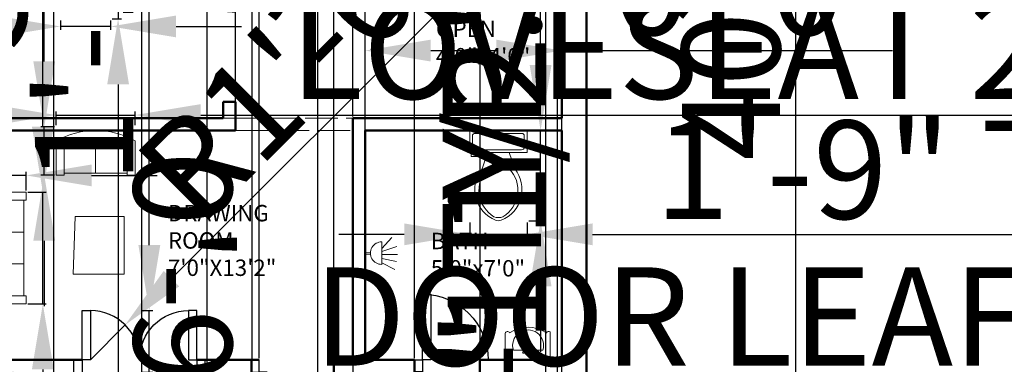
# Model space of a CAD drawing. Units: inches. Extents: x 1102 to 2414, y 295 to 1561.
# Tile 5 of 11: x 1610 to 1971, y 768 to 894. Entities that reach past the tile are written whole.
import ezdxf

# ---------------------------------------------------------------- set-up
doc = ezdxf.new("R2010")
doc.units = ezdxf.units.IN
doc.linetypes.add('ACAD_ISO02W100', pattern=[15, 12, -3])
for name, color, linetype, lineweight in [('A-ANNO-DIMS', 2, 'Continuous', 18), ('A-AREA-IDEN', 7, 'Continuous', 25), ('A-DOOR', 4, 'Continuous', 25), ('A-FLOR-FIXT', 9, 'Continuous', 18), ('A-FURN', 8, 'Continuous', 18), ('A-WALL', 7, 'Continuous', 50), ('A-WALL-OVHD', 7, 'ACAD_ISO02W100', 18)]:
    doc.layers.add(name, color=color, linetype=linetype, lineweight=lineweight)
doc.styles.get("Standard").update_dxf_attribs({"font": 'arial.ttf'})
doc.dimstyles.new('ISO-25', dxfattribs={"dimtxt": 36, "dimasz": 24, "dimexe": 1.25, "dimexo": 0.625, "dimtad": 1, "dimlunit": 4, "dimtxsty": 'Standard', "dimcen": 2.5, "dimadec": 0, "dimazin": 0, "dimtfac": 1, "dimtmove": 0, "dimatfit": 3, "dimfxl": 1, "dimarcsym": 0})

# ---------------------------------------------------------------- blocks, each defined once
blk = doc.blocks.new('*D3')
at = {"layer": 'A-ANNO-DIMS', "color": 0, "lineweight": -2, "transparency": 16777216}
for p, q in [((1818.17, 1116.76), (1895.42, 1116.76)), ((1894.17, 1092.76), (1894.17, 660.76)), ((1818.17, 636.76), (1895.42, 636.76))]:
    blk.add_line(p, q, dxfattribs=at)
at = {"layer": 'A-ANNO-DIMS', "color": 0, "transparency": 16777216}
for points in [[(1890.17, 1092.76), (1898.17, 1092.76), (1894.17, 1116.76)], [(1890.17, 660.76), (1898.17, 660.76), (1894.17, 636.76)]]:
    blk.add_solid(points, dxfattribs=at)
at = {"layer": 'Defpoints', "color": 0, "transparency": 16777216}
for p in [(1817.54, 1116.76), (1817.54, 636.76), (1894.17, 636.76)]:
    blk.add_point(p, dxfattribs=at)
at = {"layer": 'A-ANNO-DIMS', "color": 0, "transparency": 16777216, "insert": (1875.16, 876.76), "char_height": 36, "attachment_point": 5, "rotation": 90}
blk.add_mtext("40'", dxfattribs=at)
blk = doc.blocks.new('Sofa - Roundback 7 ft.')
for p, q in [((-12.00002, -32.4421), (-12.00003, -6.5971)), ((11.99997, -32.4421), (11.99998, -6.5971)), ((-36.000027, -34), (-36.000027, -11.4696)), ((-35.999844, -13.3819), (35.9998, -13.3819)), ((35.99998, -34), (35.99998, -11.4696)), ((-36.000027, -32.4421), (35.99998, -32.4421))]:
    blk.add_line(p, q)
for points in [[(-36.000027, -34), (-42.000027, -34), (-42.000027, -8)], [(41.99998, -8), (41.99998, -34), (35.99998, -34)]]:
    blk.add_lwpolyline(points)
for centre, radius, start, end in [((0, -114.25), 114.25, 68.43141, 111.5686), ((-0.00001, -127.1968), 121.1968, 72.72033, 107.2797)]:
    blk.add_arc(centre, radius, start, end)
blk = doc.blocks.new('Sofa - Roundback Loveseat 5 ft.')
for p, q in [((0, -32.44198), (0, -5.99998)), ((-24, -33.99998), (-24, -11.46958)), ((-23.9998, -13.38178), (23.99986, -13.38178)), ((24.00004, -33.99998), (24.00004, -11.46958)), ((-24, -32.44198), (24.00004, -32.44198))]:
    blk.add_line(p, q)
for points in [[(-24, -33.99998), (-30, -33.99998), (-30, -7.99998)], [(30.00004, -7.99998), (30.00004, -33.99998), (24.00004, -33.99998)]]:
    blk.add_lwpolyline(points)
for centre, radius, start, end in [((0, -60.24998), 60.24998, 60.13715, 119.8628), ((0, -61.38438), 55.38444, 64.32083, 115.6792)]:
    blk.add_arc(centre, radius, start, end)
blk = doc.blocks.new('Toilet - top')
for p, q in [((9.5, -6), (9.5, -2)), ((-10, -8.5), (-8, -8.5)), ((-10, -9.5), (-10, -8.5)), ((-7, -9.5), (-10, -9.5)), ((-8, -8.5), (-8, -8)), ((-7, -8), (-7, -9.5)), ((-4, -8), (-6, -14)), ((4, -8), (6, -14)), ((4, -14), (-4, -14))]:
    blk.add_line(p, q)
blk.add_lwpolyline([(10.5, -8), (10.5, 0), (-10.5, 0), (-10.5, -8)], close=True)
for points in [[(-9.5, -2), (-9.5, -6)], [(8.5, -1), (-8.5, -1)], [(-8.5, -7), (8.5, -7)]]:
    blk.add_lwpolyline(points)
for centre, radius, start, end in [((-8.62, -1.88), 0.884, 81.8699, 188.1301), ((8.62, -1.88), 0.884, 351.8699, 98.1301), ((-8.62, -6.12), 0.884, 171.8699, 278.1301), ((8.62, -6.12), 0.884, 261.8699, 8.1301), ((3.52, -21.58), 12.17, 141.4691, 247.9714), ((4.2, -21.82), 11.33, 136.3677, 238.9468), ((-3.52, -21.58), 12.17, 292.0284, 38.5307), ((-4.2, -21.82), 11.33, 301.053, 43.6321), ((0, -27.88), 4, 245.7318, 294.2682), ((0, -29), 4, 254.8605, 285.1395)]:
    blk.add_arc(centre, radius, start, end)
blk = doc.blocks.new('roomdoor')
for points in [[(1837.54, 1413.02), (1840.54, 1413.02), (1840.54, 1443.02), (1837.54, 1443.02)], [(1840.54, 1408.52), (1843.54, 1408.52), (1843.54, 1413.02), (1840.54, 1413.02)]]:
    blk.add_lwpolyline(points, close=True)
blk.add_arc((1840.54, 1413.02), 30, 90, 180)
blk = doc.blocks.new('utilitydoor')
for points in [[(1891.43, 1413.69), (1894.43, 1413.69), (1894.43, 1437.69), (1891.43, 1437.69)], [(1894.43, 1409.19), (1897.43, 1409.19), (1897.43, 1413.69), (1894.43, 1413.69)]]:
    blk.add_lwpolyline(points, close=True)
blk.add_arc((1894.43, 1413.69), 24, 90, 180)
blk = doc.blocks.new('DOOR-DOUBLE-LEAF-18')
blk.add_lwpolyline([(3, 22.5), (6, 22.5), (6, 4.5), (3, 4.5)], close=True)
blk.add_lwpolyline([(0, 0), (0, 4.5), (3, 4.5), (3, 0)])
blk.add_arc((6, 4.5), 18, 0, 90)
blk = doc.blocks.new('*D17')
at = {"layer": 'A-ANNO-DIMS', "color": 0, "lineweight": -2, "transparency": 16777216}
for p, q in [((1600.9, 891.85), (1102.3, 891.8)), ((1624.9, 893.98), (1624.9, 890.6)), ((1643.27, 891.85), (1624.9, 891.85)), ((1643.27, 893.98), (1643.27, 890.6)), ((1667.27, 891.85), (1691.27, 891.85))]:
    blk.add_line(p, q, dxfattribs=at)
at = {"layer": 'A-ANNO-DIMS', "color": 0, "transparency": 16777216}
for points in [[(1600.9, 895.85), (1600.9, 887.85), (1624.9, 891.85)], [(1667.27, 895.85), (1667.27, 887.85), (1643.27, 891.85)]]:
    blk.add_solid(points, dxfattribs=at)
at = {"layer": 'Defpoints', "color": 0, "transparency": 16777216}
for p in [(1624.9, 894.6), (1643.27, 894.6), (1624.9, 891.85)]:
    blk.add_point(p, dxfattribs=at)
at = {"layer": 'A-ANNO-DIMS', "color": 0, "transparency": 16777216, "insert": (1339.6, 911.06), "char_height": 36, "attachment_point": 5, "rotation": 0.0057}
blk.add_mtext('CHAIR 1\'-6 1/2" TYP.', dxfattribs=at)
blk = doc.blocks.new('*D18')
at = {"layer": 'A-ANNO-DIMS', "color": 0, "lineweight": -2, "transparency": 16777216}
for p, q in [((1646.02, 927.81), (1646.02, 951.81)), ((1643.89, 903.81), (1647.27, 903.81)), ((1646.02, 903.81), (1646.02, 894.61)), ((1643.89, 894.6), (1647.27, 894.61)), ((1646.03, 870.61), (1646.05, 625.92))]:
    blk.add_line(p, q, dxfattribs=at)
at = {"layer": 'A-ANNO-DIMS', "color": 0, "transparency": 16777216}
for points in [[(1650.02, 927.81), (1642.02, 927.81), (1646.02, 903.81)], [(1650.03, 870.61), (1642.03, 870.6), (1646.02, 894.61)]]:
    blk.add_solid(points, dxfattribs=at)
at = {"layer": 'Defpoints', "color": 0, "transparency": 16777216}
for p in [(1643.27, 903.81), (1643.27, 894.6), (1646.02, 894.61)]:
    blk.add_point(p, dxfattribs=at)
at = {"layer": 'A-ANNO-DIMS', "color": 0, "transparency": 16777216, "insert": (1665.05, 736.26), "char_height": 36, "attachment_point": 5, "rotation": 270.0057}
blk.add_mtext('0\'-9" TYP.', dxfattribs=at)
blk = doc.blocks.new('*D20')
at = {"layer": 'A-ANNO-DIMS', "color": 0, "lineweight": -2, "transparency": 16777216}
for p, q in [((1808.58, 695.77), (1808.58, 1020.95)), ((1806.65, 671.77), (1809.83, 671.77)), ((1808.58, 658.48), (1808.58, 671.77)), ((1806.65, 658.48), (1809.83, 658.48)), ((1808.58, 634.48), (1808.58, 610.48))]:
    blk.add_line(p, q, dxfattribs=at)
at = {"layer": 'A-ANNO-DIMS', "color": 0, "transparency": 16777216}
for points in [[(1804.58, 695.77), (1812.58, 695.77), (1808.58, 671.77)], [(1804.58, 634.48), (1812.58, 634.48), (1808.58, 658.48)]]:
    blk.add_solid(points, dxfattribs=at)
at = {"layer": 'Defpoints', "color": 0, "transparency": 16777216}
for p in [(1806.03, 671.77), (1808.58, 671.77), (1806.03, 658.48)]:
    blk.add_point(p, dxfattribs=at)
at = {"layer": 'A-ANNO-DIMS', "color": 0, "transparency": 16777216, "insert": (1789.34, 870.36), "char_height": 36, "attachment_point": 5, "rotation": 90}
blk.add_mtext('1\'-1 1/2" TYP.', dxfattribs=at)
blk = doc.blocks.new('*D21')
at = {"layer": 'A-ANNO-DIMS', "color": 0, "lineweight": -2, "transparency": 16777216}
for p, q in [((1731.22, 677.69), (1731.22, 665.84)), ((1806.03, 677.69), (1806.03, 665.84)), ((1755.22, 667.09), (1782.03, 667.09)), ((1806.03, 667.09), (2237.1, 667.09))]:
    blk.add_line(p, q, dxfattribs=at)
at = {"layer": 'A-ANNO-DIMS', "color": 0, "transparency": 16777216}
for points in [[(1755.22, 671.09), (1755.22, 663.09), (1731.22, 667.09)], [(1782.03, 671.09), (1782.03, 663.09), (1806.03, 667.09)]]:
    blk.add_solid(points, dxfattribs=at)
at = {"layer": 'Defpoints', "color": 0, "transparency": 16777216}
for p in [(1731.22, 678.32), (1806.03, 678.32), (1806.03, 667.09)]:
    blk.add_point(p, dxfattribs=at)
at = {"layer": 'A-ANNO-DIMS', "color": 0, "transparency": 16777216, "insert": (2033.56, 687.44), "char_height": 36, "attachment_point": 5}
blk.add_mtext('QUEEN BED 6\'-3"', dxfattribs=at)
blk = doc.blocks.new('*D24')
at = {"layer": 'A-ANNO-DIMS', "color": 0, "lineweight": -2, "transparency": 16777216}
for p, q in [((1725.17, 1080.27), (1712.37, 1080.27)), ((1713.62, 1056.27), (1713.62, 1043.39)), ((1725.17, 1019.39), (1712.37, 1019.39)), ((1713.62, 1019.39), (1713.62, 898.44))]:
    blk.add_line(p, q, dxfattribs=at)
at = {"layer": 'A-ANNO-DIMS', "color": 0, "transparency": 16777216}
for points in [[(1709.62, 1056.27), (1717.62, 1056.27), (1713.62, 1080.27)], [(1709.62, 1043.39), (1717.62, 1043.39), (1713.62, 1019.39)]]:
    blk.add_solid(points, dxfattribs=at)
at = {"layer": 'Defpoints', "color": 0, "transparency": 16777216}
for p in [(1725.8, 1080.27), (1713.62, 1019.39), (1725.8, 1019.39)]:
    blk.add_point(p, dxfattribs=at)
at = {"layer": 'A-ANNO-DIMS', "color": 0, "transparency": 16777216, "insert": (1694.62, 946.91), "char_height": 36, "attachment_point": 5, "rotation": 90}
blk.add_mtext('5\'-1"', dxfattribs=at)
blk = doc.blocks.new('*D25')
at = {"layer": 'A-ANNO-DIMS', "color": 0, "lineweight": -2, "transparency": 16777216}
for p, q in [((1800.76, 877.69), (1800.76, 1221.61)), ((1796.43, 853.69), (1802.01, 853.69)), ((1800.76, 820.65), (1800.76, 853.69)), ((1796.43, 820.65), (1802.01, 820.65)), ((1800.76, 796.65), (1800.76, 772.65))]:
    blk.add_line(p, q, dxfattribs=at)
at = {"layer": 'A-ANNO-DIMS', "color": 0, "transparency": 16777216}
for points in [[(1796.76, 877.69), (1804.76, 877.69), (1800.76, 853.69)], [(1796.76, 796.65), (1804.76, 796.65), (1800.76, 820.65)]]:
    blk.add_solid(points, dxfattribs=at)
at = {"layer": 'Defpoints', "color": 0, "transparency": 16777216}
for p in [(1795.81, 853.69), (1800.76, 853.69), (1795.81, 820.65)]:
    blk.add_point(p, dxfattribs=at)
at = {"layer": 'A-ANNO-DIMS', "color": 0, "transparency": 16777216, "insert": (1781.53, 1061.65), "char_height": 36, "attachment_point": 5, "rotation": 90}
blk.add_mtext('WC 2\'-9" TYP.', dxfattribs=at)
blk = doc.blocks.new('*D26')
at = {"layer": 'A-ANNO-DIMS', "color": 0, "lineweight": -2, "transparency": 16777216}
for p, q in [((1774.81, 820.02), (1774.81, 814.44)), ((1795.81, 820.02), (1795.81, 814.44)), ((1750.81, 815.69), (1726.81, 815.69)), ((1774.81, 815.69), (1795.81, 815.69)), ((1819.81, 815.69), (2061.11, 815.69))]:
    blk.add_line(p, q, dxfattribs=at)
at = {"layer": 'A-ANNO-DIMS', "color": 0, "transparency": 16777216}
for points in [[(1750.81, 819.69), (1750.81, 811.69), (1774.81, 815.69)], [(1819.81, 819.69), (1819.81, 811.69), (1795.81, 815.69)]]:
    blk.add_solid(points, dxfattribs=at)
at = {"layer": 'Defpoints', "color": 0, "transparency": 16777216}
for p in [(1774.81, 820.65), (1795.81, 820.65), (1795.81, 815.69)]:
    blk.add_point(p, dxfattribs=at)
at = {"layer": 'A-ANNO-DIMS', "color": 0, "transparency": 16777216, "insert": (1952.46, 834.69), "char_height": 36, "attachment_point": 5}
blk.add_mtext('1\'-9" TYP.', dxfattribs=at)
blk = doc.blocks.new('*D29')
at = {"layer": 'A-ANNO-DIMS', "color": 0, "lineweight": -2, "transparency": 16777216}
for p, q in [((1806.82, 1011.76), (1806.82, 1035.76)), ((1803.17, 987.76), (1808.07, 987.76)), ((1806.82, 987.76), (1806.82, 959.26)), ((1803.17, 959.26), (1808.07, 959.26)), ((1806.82, 935.26), (1806.82, 295.33))]:
    blk.add_line(p, q, dxfattribs=at)
at = {"layer": 'A-ANNO-DIMS', "color": 0, "transparency": 16777216}
for points in [[(1802.82, 1011.76), (1810.82, 1011.76), (1806.82, 987.76)], [(1802.82, 935.26), (1810.82, 935.26), (1806.82, 959.26)]]:
    blk.add_solid(points, dxfattribs=at)
at = {"layer": 'Defpoints', "color": 0, "transparency": 16777216}
for p in [(1802.54, 987.76), (1802.54, 959.26), (1806.82, 959.26)]:
    blk.add_point(p, dxfattribs=at)
at = {"layer": 'A-ANNO-DIMS', "color": 0, "transparency": 16777216, "insert": (1787.57, 603.3), "char_height": 36, "attachment_point": 5, "rotation": 90}
blk.add_mtext('BATH DOOR 2\'-4 1/2" TYP.', dxfattribs=at)
blk = doc.blocks.new('*D31')
at = {"layer": 'A-ANNO-DIMS', "color": 0, "lineweight": -2, "transparency": 16777216}
for p, q in [((1629.86, 764.63), (1629.86, 760.41)), ((1653.86, 764.63), (1653.86, 760.41)), ((1605.86, 761.66), (1581.86, 761.66)), ((1629.86, 761.66), (1653.86, 761.66)), ((1677.86, 761.66), (2225.36, 761.66))]:
    blk.add_line(p, q, dxfattribs=at)
at = {"layer": 'A-ANNO-DIMS', "color": 0, "transparency": 16777216}
for points in [[(1605.86, 765.66), (1605.86, 757.66), (1629.86, 761.66)], [(1677.86, 765.66), (1677.86, 757.66), (1653.86, 761.66)]]:
    blk.add_solid(points, dxfattribs=at)
at = {"layer": 'Defpoints', "color": 0, "transparency": 16777216}
for p in [(1629.86, 765.26), (1653.86, 765.26), (1653.86, 761.66)]:
    blk.add_point(p, dxfattribs=at)
at = {"layer": 'A-ANNO-DIMS', "color": 0, "transparency": 16777216, "insert": (1963.61, 780.91), "char_height": 36, "attachment_point": 5}
blk.add_mtext('DOOR LEAF 2\'-0" TYP.', dxfattribs=at)
blk = doc.blocks.new('*D32')
at = {"layer": 'A-ANNO-DIMS', "color": 0, "lineweight": -2, "transparency": 16777216}
for p, q in [((1657.46, 811.76), (1657.46, 1164.91)), ((1654.49, 787.76), (1658.71, 787.76)), ((1657.46, 765.26), (1657.46, 787.76)), ((1654.49, 765.26), (1658.71, 765.26)), ((1657.46, 741.26), (1657.46, 717.26))]:
    blk.add_line(p, q, dxfattribs=at)
at = {"layer": 'A-ANNO-DIMS', "color": 0, "transparency": 16777216}
for points in [[(1653.46, 811.76), (1661.46, 811.76), (1657.46, 787.76)], [(1653.46, 741.26), (1661.46, 741.26), (1657.46, 765.26)]]:
    blk.add_solid(points, dxfattribs=at)
at = {"layer": 'Defpoints', "color": 0, "transparency": 16777216}
for p in [(1653.86, 787.76), (1657.46, 787.76), (1653.86, 765.26)]:
    blk.add_point(p, dxfattribs=at)
at = {"layer": 'A-ANNO-DIMS', "color": 0, "transparency": 16777216, "insert": (1638.22, 1000.34), "char_height": 36, "attachment_point": 5, "rotation": 90}
blk.add_mtext('1\'-10 1/2" TYP.', dxfattribs=at)
blk = doc.blocks.new('*D37')
at = {"layer": 'A-ANNO-DIMS', "color": 0, "lineweight": -2, "transparency": 16777216}
for p, q in [((1618.46, 855.15), (1618.46, 1126.82)), ((1612.94, 831.15), (1619.71, 831.15)), ((1618.46, 790.23), (1618.46, 831.15)), ((1612.94, 790.23), (1619.71, 790.23)), ((1618.46, 766.23), (1618.46, 742.23))]:
    blk.add_line(p, q, dxfattribs=at)
at = {"layer": 'A-ANNO-DIMS', "color": 0, "transparency": 16777216}
for points in [[(1614.46, 855.15), (1622.46, 855.15), (1618.46, 831.15)], [(1614.46, 766.23), (1622.46, 766.23), (1618.46, 790.23)]]:
    blk.add_solid(points, dxfattribs=at)
at = {"layer": 'Defpoints', "color": 0, "transparency": 16777216}
for p in [(1612.32, 831.15), (1618.46, 831.15), (1612.32, 790.23)]:
    blk.add_point(p, dxfattribs=at)
at = {"layer": 'A-ANNO-DIMS', "color": 0, "transparency": 16777216, "insert": (1599.19, 1002.98), "char_height": 36, "attachment_point": 5, "rotation": 90}
blk.add_mtext('SOFA 3\'-5"', dxfattribs=at)
blk = doc.blocks.new('*D38')
at = {"layer": 'A-ANNO-DIMS', "color": 0, "lineweight": -2, "transparency": 16777216}
for p, q in [((1570.46, 837.28), (1452.9, 837.28)), ((1594.46, 831.77), (1594.46, 838.53)), ((1612.32, 837.28), (1594.46, 837.28)), ((1612.32, 831.77), (1612.32, 838.53)), ((1636.32, 837.28), (1660.32, 837.28))]:
    blk.add_line(p, q, dxfattribs=at)
at = {"layer": 'A-ANNO-DIMS', "color": 0, "transparency": 16777216}
for points in [[(1570.46, 841.28), (1570.46, 833.28), (1594.46, 837.28)], [(1636.32, 841.28), (1636.32, 833.28), (1612.32, 837.28)]]:
    blk.add_solid(points, dxfattribs=at)
at = {"layer": 'Defpoints', "color": 0, "transparency": 16777216}
for p in [(1594.46, 837.28), (1594.46, 831.15), (1612.32, 831.15)]:
    blk.add_point(p, dxfattribs=at)
at = {"layer": 'A-ANNO-DIMS', "color": 0, "transparency": 16777216, "insert": (1499.68, 856.29), "char_height": 36, "attachment_point": 5}
blk.add_mtext('1\'-6"', dxfattribs=at)
blk = doc.blocks.new('*D39')
at = {"layer": 'A-ANNO-DIMS', "color": 0, "lineweight": -2, "transparency": 16777216}
for p, q in [((1599.32, 859.39), (1575.32, 859.39)), ((1623.32, 855.67), (1623.32, 860.64)), ((1623.32, 859.39), (1652.27, 859.39)), ((1652.27, 855.67), (1652.27, 860.64)), ((1676.27, 859.39), (2075.12, 859.39))]:
    blk.add_line(p, q, dxfattribs=at)
at = {"layer": 'A-ANNO-DIMS', "color": 0, "transparency": 16777216}
for points in [[(1599.32, 863.39), (1599.32, 855.39), (1623.32, 859.39)], [(1676.27, 863.39), (1676.27, 855.39), (1652.27, 859.39)]]:
    blk.add_solid(points, dxfattribs=at)
at = {"layer": 'Defpoints', "color": 0, "transparency": 16777216}
for p in [(1652.27, 859.39), (1623.32, 855.05), (1652.27, 855.05)]:
    blk.add_point(p, dxfattribs=at)
at = {"layer": 'A-ANNO-DIMS', "color": 0, "transparency": 16777216, "insert": (1887.69, 878.64), "char_height": 36, "attachment_point": 5}
blk.add_mtext('LOVESEAT 2\'-5"', dxfattribs=at)
blk = doc.blocks.new('*D40')
at = {"layer": 'A-ANNO-DIMS', "color": 0, "lineweight": -2, "transparency": 16777216}
for p, q in [((1618.98, 879.05), (1618.98, 1080.49)), ((1622.7, 855.05), (1617.73, 855.05)), ((1618.98, 837.36), (1618.98, 855.05)), ((1622.7, 837.36), (1617.73, 837.36)), ((1618.98, 813.36), (1618.98, 789.36))]:
    blk.add_line(p, q, dxfattribs=at)
at = {"layer": 'A-ANNO-DIMS', "color": 0, "transparency": 16777216}
for points in [[(1614.98, 879.05), (1622.98, 879.05), (1618.98, 855.05)], [(1614.98, 813.36), (1622.98, 813.36), (1618.98, 837.36)]]:
    blk.add_solid(points, dxfattribs=at)
at = {"layer": 'Defpoints', "color": 0, "transparency": 16777216}
for p in [(1618.98, 855.05), (1623.32, 855.05), (1623.32, 837.36)]:
    blk.add_point(p, dxfattribs=at)
at = {"layer": 'A-ANNO-DIMS', "color": 0, "transparency": 16777216, "insert": (1599.74, 991.77), "char_height": 36, "attachment_point": 5, "rotation": 90}
blk.add_mtext('1\'-5 1/2"', dxfattribs=at)
blk = doc.blocks.new('*D45')
at = {"layer": 'A-ANNO-DIMS', "color": 0, "lineweight": -2, "transparency": 16777216}
for p, q in [((1736.54, 770.38), (1736.54, 1147.26)), ((1754.54, 770.38), (1754.54, 1147.26)), ((1712.54, 1146.01), (1688.54, 1146.01)), ((1736.54, 1146.01), (1754.54, 1146.01)), ((1778.54, 1146.01), (1896.1, 1146.01))]:
    blk.add_line(p, q, dxfattribs=at)
at = {"layer": 'A-ANNO-DIMS', "color": 0, "transparency": 16777216}
for points in [[(1712.54, 1150.01), (1712.54, 1142.01), (1736.54, 1146.01)], [(1778.54, 1150.01), (1778.54, 1142.01), (1754.54, 1146.01)]]:
    blk.add_solid(points, dxfattribs=at)
at = {"layer": 'Defpoints', "color": 0, "transparency": 16777216}
for p in [(1754.54, 1146.01), (1736.54, 769.76), (1754.54, 769.76)]:
    blk.add_point(p, dxfattribs=at)
at = {"layer": 'A-ANNO-DIMS', "color": 0, "transparency": 16777216, "insert": (1849.32, 1165.02), "char_height": 36, "attachment_point": 5}
blk.add_mtext('1\'-6"', dxfattribs=at)
blk = doc.blocks.new('*D46')
at = {"layer": 'A-ANNO-DIMS', "color": 0, "lineweight": -2, "transparency": 16777216}
for p, q in [((1732.04, 857.63), (1732.04, 606.26)), ((1586.54, 853.13), (1586.54, 606.26)), ((1610.54, 607.51), (1708.04, 607.51)), ((1732.04, 607.51), (1961.46, 607.51))]:
    blk.add_line(p, q, dxfattribs=at)
at = {"layer": 'A-ANNO-DIMS', "color": 0, "transparency": 16777216}
for points in [[(1610.54, 611.51), (1610.54, 603.51), (1586.54, 607.51)], [(1708.04, 611.51), (1708.04, 603.51), (1732.04, 607.51)]]:
    blk.add_solid(points, dxfattribs=at)
at = {"layer": 'Defpoints', "color": 0, "transparency": 16777216}
for p in [(1732.04, 858.26), (1586.54, 853.76), (1732.04, 607.51)]:
    blk.add_point(p, dxfattribs=at)
at = {"layer": 'A-ANNO-DIMS', "color": 0, "transparency": 16777216, "insert": (1858.75, 626.75), "char_height": 36, "attachment_point": 5}
blk.add_mtext('12\'-1 1/2"', dxfattribs=at)
blk = doc.blocks.new('*D47')
at = {"layer": 'A-ANNO-DIMS', "color": 0, "lineweight": -2, "transparency": 16777216}
for p, q in [((1736.54, 854.38), (1736.54, 884.26)), ((1808.54, 854.38), (1808.54, 884.26)), ((1760.54, 883.01), (1784.54, 883.01)), ((1808.54, 883.01), (1929.69, 883.01))]:
    blk.add_line(p, q, dxfattribs=at)
at = {"layer": 'A-ANNO-DIMS', "color": 0, "transparency": 16777216}
for points in [[(1760.54, 887.01), (1760.54, 879.01), (1736.54, 883.01)], [(1784.54, 887.01), (1784.54, 879.01), (1808.54, 883.01)]]:
    blk.add_solid(points, dxfattribs=at)
at = {"layer": 'Defpoints', "color": 0, "transparency": 16777216}
for p in [(1808.54, 883.01), (1736.54, 853.76), (1808.54, 853.76)]:
    blk.add_point(p, dxfattribs=at)
at = {"layer": 'A-ANNO-DIMS', "color": 0, "transparency": 16777216, "insert": (1881.12, 902.02), "char_height": 36, "attachment_point": 5}
blk.add_mtext('6\'-0"', dxfattribs=at)
blk = doc.blocks.new('*D48')
at = {"layer": 'A-ANNO-DIMS', "color": 0, "lineweight": -2, "transparency": 16777216}
for p, q in [((1689.04, 854.38), (1689.04, 1147.26)), ((1732.04, 858.88), (1732.04, 1147.26)), ((1665.04, 1146.01), (1641.04, 1146.01)), ((1689.04, 1146.01), (1732.04, 1146.01)), ((1756.04, 1146.01), (1876.97, 1146.01))]:
    blk.add_line(p, q, dxfattribs=at)
at = {"layer": 'A-ANNO-DIMS', "color": 0, "transparency": 16777216}
for points in [[(1665.04, 1150.01), (1665.04, 1142.01), (1689.04, 1146.01)], [(1756.04, 1150.01), (1756.04, 1142.01), (1732.04, 1146.01)]]:
    blk.add_solid(points, dxfattribs=at)
at = {"layer": 'Defpoints', "color": 0, "transparency": 16777216}
for p in [(1732.04, 1146.01), (1732.04, 858.26), (1689.04, 853.76)]:
    blk.add_point(p, dxfattribs=at)
at = {"layer": 'A-ANNO-DIMS', "color": 0, "transparency": 16777216, "insert": (1828.51, 1165.03), "char_height": 36, "attachment_point": 5}
blk.add_mtext('3\'-7"', dxfattribs=at)
blk = doc.blocks.new('*D50')
at = {"layer": 'A-ANNO-DIMS', "color": 0, "lineweight": -2, "transparency": 16777216}
for p, q in [((1586.54, 987.13), (1586.54, 606.26)), ((1654.54, 987.13), (1654.54, 606.26)), ((1610.54, 607.51), (1630.54, 607.51)), ((1654.54, 607.51), (1775.49, 607.51))]:
    blk.add_line(p, q, dxfattribs=at)
at = {"layer": 'A-ANNO-DIMS', "color": 0, "transparency": 16777216}
for points in [[(1610.54, 611.51), (1610.54, 603.51), (1586.54, 607.51)], [(1630.54, 611.51), (1630.54, 603.51), (1654.54, 607.51)]]:
    blk.add_solid(points, dxfattribs=at)
at = {"layer": 'Defpoints', "color": 0, "transparency": 16777216}
for p in [(1586.54, 987.76), (1654.54, 987.76), (1654.54, 607.51)]:
    blk.add_point(p, dxfattribs=at)
at = {"layer": 'A-ANNO-DIMS', "color": 0, "transparency": 16777216, "insert": (1727.02, 626.52), "char_height": 36, "attachment_point": 5}
blk.add_mtext('5\'-8"', dxfattribs=at)
blk = doc.blocks.new('*D55')
at = {"layer": 'A-ANNO-DIMS', "color": 0, "lineweight": -2, "transparency": 16777216}
for p, q in [((1586.54, 722.38), (1586.54, 1147.26)), ((1622.54, 722.38), (1622.54, 1147.26)), ((1562.54, 1146.01), (1538.54, 1146.01)), ((1586.54, 1146.01), (1622.54, 1146.01)), ((1646.54, 1146.01), (1767.47, 1146.01))]:
    blk.add_line(p, q, dxfattribs=at)
at = {"layer": 'A-ANNO-DIMS', "color": 0, "transparency": 16777216}
for points in [[(1562.54, 1150.01), (1562.54, 1142.01), (1586.54, 1146.01)], [(1646.54, 1150.01), (1646.54, 1142.01), (1622.54, 1146.01)]]:
    blk.add_solid(points, dxfattribs=at)
at = {"layer": 'Defpoints', "color": 0, "transparency": 16777216}
for p in [(1622.54, 1146.01), (1586.54, 721.76), (1622.54, 721.76)]:
    blk.add_point(p, dxfattribs=at)
at = {"layer": 'A-ANNO-DIMS', "color": 0, "transparency": 16777216, "insert": (1719.01, 1165.03), "char_height": 36, "attachment_point": 5}
blk.add_mtext('3\'-0"', dxfattribs=at)
blk = doc.blocks.new('*D59')
at = {"layer": 'A-ANNO-DIMS', "color": 0, "lineweight": -2, "transparency": 16777216}
for p, q in [((1548.29, 962.66), (1548.29, 1112.19)), ((1612.15, 938.66), (1547.04, 938.66)), ((1548.29, 903.8), (1548.29, 938.66)), ((1612.15, 903.8), (1547.04, 903.8)), ((1548.29, 879.8), (1548.29, 855.8))]:
    blk.add_line(p, q, dxfattribs=at)
at = {"layer": 'A-ANNO-DIMS', "color": 0, "transparency": 16777216}
for points in [[(1544.29, 962.66), (1552.29, 962.66), (1548.29, 938.66)], [(1544.29, 879.8), (1552.29, 879.8), (1548.29, 903.8)]]:
    blk.add_solid(points, dxfattribs=at)
at = {"layer": 'Defpoints', "color": 0, "transparency": 16777216}
for p in [(1548.29, 938.66), (1612.78, 938.66), (1612.78, 903.8)]:
    blk.add_point(p, dxfattribs=at)
at = {"layer": 'A-ANNO-DIMS', "color": 0, "transparency": 16777216, "insert": (1529.6, 1049.43), "char_height": 36, "attachment_point": 5, "rotation": 90}
blk.add_mtext('2\'-11"', dxfattribs=at)
blk = doc.blocks.new('*D62')
at = {"layer": 'A-ANNO-DIMS', "color": 0, "lineweight": -2, "transparency": 16777216}
for p, q in [((1778.54, 982.63), (1778.54, 606.26)), ((1802.54, 982.63), (1802.54, 606.26)), ((1754.54, 607.51), (1730.54, 607.51)), ((1778.54, 607.51), (1802.54, 607.51)), ((1826.54, 607.51), (1948.11, 607.51))]:
    blk.add_line(p, q, dxfattribs=at)
at = {"layer": 'A-ANNO-DIMS', "color": 0, "transparency": 16777216}
for points in [[(1754.54, 611.51), (1754.54, 603.51), (1778.54, 607.51)], [(1826.54, 611.51), (1826.54, 603.51), (1802.54, 607.51)]]:
    blk.add_solid(points, dxfattribs=at)
at = {"layer": 'Defpoints', "color": 0, "transparency": 16777216}
for p in [(1778.54, 983.26), (1802.54, 983.26), (1802.54, 607.51)]:
    blk.add_point(p, dxfattribs=at)
at = {"layer": 'A-ANNO-DIMS', "color": 0, "transparency": 16777216, "insert": (1899.32, 626.52), "char_height": 36, "attachment_point": 5}
blk.add_mtext('2\'-0"', dxfattribs=at)
blk = doc.blocks.new('*D63')
at = {"layer": 'A-ANNO-DIMS', "color": 0, "lineweight": -2, "transparency": 16777216}
for p, q in [((1654.54, 982.63), (1654.54, 606.26)), ((1678.54, 982.63), (1678.54, 606.26)), ((1630.54, 607.51), (1606.54, 607.51)), ((1654.54, 607.51), (1678.54, 607.51)), ((1702.54, 607.51), (1824.11, 607.51))]:
    blk.add_line(p, q, dxfattribs=at)
at = {"layer": 'A-ANNO-DIMS', "color": 0, "transparency": 16777216}
for points in [[(1630.54, 611.51), (1630.54, 603.51), (1654.54, 607.51)], [(1702.54, 611.51), (1702.54, 603.51), (1678.54, 607.51)]]:
    blk.add_solid(points, dxfattribs=at)
at = {"layer": 'Defpoints', "color": 0, "transparency": 16777216}
for p in [(1654.54, 983.26), (1678.54, 983.26), (1678.54, 607.51)]:
    blk.add_point(p, dxfattribs=at)
at = {"layer": 'A-ANNO-DIMS', "color": 0, "transparency": 16777216, "insert": (1775.32, 626.52), "char_height": 36, "attachment_point": 5}
blk.add_mtext('2\'-0"', dxfattribs=at)
blk = doc.blocks.new('*D64')
at = {"layer": 'A-ANNO-DIMS', "color": 0, "lineweight": -2, "transparency": 16777216}
for p, q in [((1695.04, 982.63), (1695.04, 606.26)), ((1719.04, 982.63), (1719.04, 606.26)), ((1671.04, 607.51), (1647.04, 607.51)), ((1695.04, 607.51), (1719.04, 607.51)), ((1743.04, 607.51), (1864.61, 607.51))]:
    blk.add_line(p, q, dxfattribs=at)
at = {"layer": 'A-ANNO-DIMS', "color": 0, "transparency": 16777216}
for points in [[(1671.04, 611.51), (1671.04, 603.51), (1695.04, 607.51)], [(1743.04, 611.51), (1743.04, 603.51), (1719.04, 607.51)]]:
    blk.add_solid(points, dxfattribs=at)
at = {"layer": 'Defpoints', "color": 0, "transparency": 16777216}
for p in [(1695.04, 983.26), (1719.04, 983.26), (1719.04, 607.51)]:
    blk.add_point(p, dxfattribs=at)
at = {"layer": 'A-ANNO-DIMS', "color": 0, "transparency": 16777216, "insert": (1815.82, 626.52), "char_height": 36, "attachment_point": 5}
blk.add_mtext('2\'-0"', dxfattribs=at)
blk = doc.blocks.new('*D65')
at = {"layer": 'A-ANNO-DIMS', "color": 0, "lineweight": -2, "transparency": 16777216}
for p, q in [((1697.64, 770.38), (1697.64, 1147.26)), ((1725.04, 770.38), (1725.04, 1147.26)), ((1673.64, 1146.01), (1649.64, 1146.01)), ((1697.64, 1146.01), (1725.04, 1146.01)), ((1749.04, 1146.01), (1954.49, 1146.01))]:
    blk.add_line(p, q, dxfattribs=at)
at = {"layer": 'A-ANNO-DIMS', "color": 0, "transparency": 16777216}
for points in [[(1673.64, 1150.01), (1673.64, 1142.01), (1697.64, 1146.01)], [(1749.04, 1150.01), (1749.04, 1142.01), (1725.04, 1146.01)]]:
    blk.add_solid(points, dxfattribs=at)
at = {"layer": 'Defpoints', "color": 0, "transparency": 16777216}
for p in [(1725.04, 1146.01), (1697.64, 769.76), (1725.04, 769.76)]:
    blk.add_point(p, dxfattribs=at)
at = {"layer": 'A-ANNO-DIMS', "color": 0, "transparency": 16777216, "insert": (1863.77, 1165.26), "char_height": 36, "attachment_point": 5}
blk.add_mtext('2\'-3 1/2"', dxfattribs=at)
blk = doc.blocks.new('*D69')
at = {"layer": 'A-ANNO-DIMS', "color": 0, "lineweight": -2, "transparency": 16777216}
for p, q in [((1775.45, 909.34), (1665.56, 799.46)), ((1635.86, 769.76), (1648.59, 782.49))]:
    blk.add_line(p, q, dxfattribs=at)
at = {"layer": 'A-ANNO-DIMS', "color": 0, "transparency": 16777216}
blk.add_solid([(1662.73, 802.29), (1668.39, 796.63), (1648.59, 782.49)], dxfattribs=at)
at = {"layer": 'Defpoints', "color": 0, "transparency": 16777216}
for p in [(1648.59, 782.49), (1635.86, 769.76)]:
    blk.add_point(p, dxfattribs=at)
at = {"layer": 'A-ANNO-DIMS', "color": 0, "transparency": 16777216, "insert": (1715.55, 876.32), "char_height": 36, "attachment_point": 5, "rotation": 45}
blk.add_mtext('R1\'-6"', dxfattribs=at)

msp = doc.modelspace()

# ---------------------------------------------------------------- linework, layer by layer
at = {"layer": 'A-FLOR-FIXT'}
for p, q in [((1742.618, 810.56), (1746.255, 814.541)), ((1742.618, 812.925), (1742.618, 804.685)), ((1736.544, 808.967), (1738.415, 808.917)), ((1736.544, 808.33), (1738.426, 808.48)), ((1742.618, 809.445), (1748.136, 811.293)), ((1742.618, 808.362), (1748.359, 808.33)), ((1742.618, 806.865), (1748.009, 805.687)), ((1742.618, 805.273), (1747.339, 802.82)), ((1787.777, 769.76), (1787.777, 779.467)), ((1804.289, 769.76), (1804.289, 779.929)), ((1790.827, 773.205), (1801.552, 773.205)), ((1787.777, 769.76), (1804.289, 769.76))]:
    msp.add_line(p, q, dxfattribs=at)
for centre, radius in [((1794.411, 772.402), 0.284), ((1796.037, 774.2), 0.461), ((1796.032, 772.706), 0.365), ((1797.572, 772.199), 0.324)]:
    msp.add_circle(centre, radius, dxfattribs=at)
for centre, radius, start, end in [((1742.534, 808.805), 4.121, 88.83988, 271.16012), ((1788.596, 779.214), 0.857, 25.5147, 162.79987), ((1796.17, 769.344), 12.292, 56.40939, 123.59061), ((1796.189, 774.997), 5.654, 341.51851, 198.48149), ((1803.736, 779.351), 0.8, 46.25991, 163.17544)]:
    msp.add_arc(centre, radius, start, end, dxfattribs=at)
at = {"layer": 'A-FURN'}
for p, q in [((1629.594, 801.128), (1630.276, 822.247)), ((1630.276, 822.247), (1648.23, 822.247)), ((1648.23, 822.247), (1648.23, 801.128)), ((1648.23, 801.128), (1629.594, 801.128))]:
    msp.add_line(p, q, dxfattribs=at)
at = {"layer": 'A-WALL'}
for p, q in [((1817.544, 636.76), (1817.544, 1116.76)), ((1808.544, 858.26), (1808.544, 906.26)), ((1684.544, 864.26), (1684.544, 858.26)), ((1684.544, 858.26), (1684.544, 864.26)), ((1684.544, 864.26), (1689.044, 864.26)), ((1689.044, 864.26), (1689.044, 853.76)), ((1684.544, 858.26), (1586.544, 858.26)), ((1808.544, 858.26), (1732.044, 858.26)), ((1732.044, 769.76), (1732.044, 858.26)), ((1689.044, 853.76), (1586.544, 853.76)), ((1808.544, 853.76), (1736.544, 853.76)), ((1736.544, 769.76), (1736.544, 853.76)), ((1808.544, 769.76), (1808.544, 853.76)), ((1632.864, 769.76), (1586.544, 769.76)), ((1684.544, 769.76), (1674.864, 769.76)), ((1689.044, 769.76), (1674.864, 769.76)), ((1689.044, 769.76), (1697.644, 769.76)), ((1697.644, 769.76), (1689.044, 769.76)), ((1744.044, 769.76), (1725.044, 769.76)), ((1725.044, 769.76), (1725.044, 765.26)), ((1736.544, 769.76), (1754.544, 769.76)), ((1754.544, 769.76), (1748.544, 769.76)), ((1754.544, 769.76), (1754.544, 765.26)), ((1808.544, 769.76), (1778.544, 769.76)), ((1778.544, 769.76), (1778.544, 765.26))]:
    msp.add_line(p, q, dxfattribs=at)
at = {"layer": 'A-WALL-OVHD'}
for p, q in [((1684.544, 858.26), (1732.044, 858.26)), ((1689.044, 853.76), (1732.044, 853.76))]:
    msp.add_line(p, q, dxfattribs=at)

# ---------------------------------------------------------------- block references
at = {"layer": 'A-DOOR', "xscale": -1}
msp.add_blockref('utilitydoor', (3651.978, -643.928), dxfattribs=at)
at = {"layer": 'A-DOOR'}
msp.add_blockref('DOOR-DOUBLE-LEAF-18', (1629.864, 765.26), dxfattribs=at)
at = {"layer": 'A-DOOR', "extrusion": (0, 0, -1), "zscale": -1}
msp.add_blockref('DOOR-DOUBLE-LEAF-18', (-1677.863, 765.26), dxfattribs=at)
at = {"layer": 'A-DOOR', "rotation": 180}
msp.add_blockref('roomdoor', (3538.188, 2178.278), dxfattribs=at)
at = {"layer": 'A-FLOR-FIXT'}
msp.add_blockref('Toilet - top', (1785.307, 853.692), dxfattribs=at)
at = {"layer": 'A-FURN', "xscale": 0.4824574757024864, "yscale": 0.4824574757024864, "zscale": 0.4824574757024864}
msp.add_blockref('Sofa - Roundback Loveseat 5 ft.', (1637.794, 853.76), dxfattribs=at)
at = {"layer": 'A-FURN', "xscale": 0.4870553998389214, "yscale": 0.4870553998389214, "zscale": 0.4870553998389214, "rotation": 90}
msp.add_blockref('Sofa - Roundback 7 ft.', (1595.759, 810.689), dxfattribs=at)

# ---------------------------------------------------------------- texts
at = {"layer": 'A-AREA-IDEN', "char_height": 6, "attachment_point": 1}
for s, insert in [('OPEN\\P4\'0"x4\'0"', (1762.445, 893.945)), ('DRAWING ROOM\\P7\'0"X13\'2"', (1664.274, 826.458)), ('BATH\\P5\'0"x7\'0"', (1760.547, 816.257))]:
    msp.add_mtext_dynamic_manual_height_columns(s, width=50.64919, gutter_width=12.5, heights=[0], dxfattribs=dict(at, insert=insert))

# ---------------------------------------------------------------- dimensions: what is measured, and where the dimension line sits
at = {"layer": 'A-ANNO-DIMS'}
for base, p1, p2, picture, middle in [((1725.044, 1146.01), (1697.644, 769.76), (1725.044, 769.76), '*D65', (1863.767, 1165.261)), ((1622.544, 1146.01), (1586.544, 721.76), (1622.544, 721.76), '*D55', (1719.005, 1165.028)), ((1732.044, 1146.01), (1689.044, 853.76), (1732.044, 858.26), '*D48', (1828.505, 1165.028)), ((1754.544, 1146.01), (1736.544, 769.76), (1754.544, 769.76), '*D45', (1849.323, 1165.015)), ((1654.544, 607.51), (1586.544, 987.76), (1654.544, 987.76), '*D50', (1727.018, 626.515)), ((1678.544, 607.51), (1654.544, 983.26), (1678.544, 983.26), '*D63', (1775.325, 626.515)), ((1719.044, 607.51), (1695.044, 983.26), (1719.044, 983.26), '*D64', (1815.825, 626.515)), ((1802.544, 607.51), (1778.544, 983.26), (1802.544, 983.26), '*D62', (1899.325, 626.515)), ((1808.544, 883.01), (1736.544, 853.76), (1808.544, 853.76), '*D47', (1881.116, 902.015)), ((1732.044, 607.51), (1586.544, 853.76), (1732.044, 858.26), '*D46', (1858.751, 626.749))]:
    dim = msp.add_linear_dim(base=base, p1=p1, p2=p2, dimstyle='ISO-25', override={"dimdec": 1, "dimlfac": 1, "dimrnd": 0, "dimzin": 1, "dimdsep": 46, "dimlunit": 4, "dimfrac": 2}, dxfattribs=at)
    dim.commit()
    dim.dimension.update_dxf_attribs({"geometry": picture, "text_midpoint": middle})
for base, p1, p2, angle, text, picture, middle in [((1800.764, 853.692), (1795.807, 820.646), (1795.807, 853.692), 90, 'WC <> TYP.', '*D25', (1781.525, 1061.653)), ((1657.464, 787.76), (1653.864, 765.26), (1653.864, 787.76), 90, '<> TYP.', '*D32', (1638.225, 1000.337)), ((1618.456, 831.145), (1612.319, 790.233), (1612.319, 831.145), 90, 'SOFA <>', '*D37', (1599.192, 1002.983)), ((1806.819, 959.26), (1802.544, 987.76), (1802.544, 959.26), 270, 'BATH DOOR <> TYP.', '*D29', (1787.568, 603.296)), ((1624.9, 891.848), (1643.269, 894.605), (1624.9, 894.603), 180.00567, 'CHAIR <> TYP.', '*D17', (1339.596, 911.058)), ((1808.577, 671.77), (1806.028, 658.482), (1806.028, 671.77), 90, '<> TYP.', '*D20', (1789.338, 870.362)), ((1646.024, 894.605), (1643.268, 903.806), (1643.269, 894.605), 270.00567, '<> TYP.', '*D18', (1665.045, 736.263))]:
    dim = msp.add_linear_dim(base=base, p1=p1, p2=p2, angle=angle, text=text, dimstyle='ISO-25', override={"dimdec": 1, "dimlfac": 1, "dimrnd": 0, "dimzin": 1, "dimdsep": 46, "dimlunit": 4, "dimfrac": 2}, dxfattribs=at)
    dim.commit()
    dim.dimension.update_dxf_attribs({"geometry": picture, "text_midpoint": middle})
for base, p1, p2, angle, picture, middle in [((1548.294, 938.663), (1612.778, 903.803), (1612.778, 938.663), 90, '*D59', (1529.595, 1049.429)), ((1618.978, 855.046), (1623.32, 837.356), (1623.32, 855.046), 90, '*D40', (1599.739, 991.768)), ((1713.621, 1019.387), (1725.798, 1080.268), (1725.798, 1019.387), 270, '*D24', (1694.616, 946.913)), ((1594.46, 837.282), (1612.319, 831.145), (1594.46, 831.145), 180, '*D38', (1499.681, 856.288))]:
    dim = msp.add_linear_dim(base=base, p1=p1, p2=p2, angle=angle, dimstyle='ISO-25', override={"dimdec": 1, "dimlfac": 1, "dimrnd": 0, "dimzin": 1, "dimdsep": 46, "dimlunit": 4, "dimfrac": 2}, dxfattribs=at)
    dim.commit()
    dim.dimension.update_dxf_attribs({"geometry": picture, "text_midpoint": middle})
dim = msp.add_linear_dim(base=(1894.167, 636.76), p1=(1817.544, 1116.76), p2=(1817.544, 636.76), angle=90, dimstyle='ISO-25', override={"dimclrd": 0, "dimclre": 0, "dimclrt": 0}, dxfattribs=at)
dim.commit()
dim.dimension.update_dxf_attribs({"geometry": '*D3', "text_midpoint": (1894.167, 876.76), "dimtype": 160})
dim = msp.add_radius_dim(center=(1635.864, 769.76), mpoint=(1648.592, 782.488), dimstyle='ISO-25', override={"dimdec": 1, "dimlfac": 1, "dimrnd": 0, "dimzin": 1, "dimdsep": 46, "dimlunit": 4, "dimfrac": 2}, dxfattribs=at)
dim.commit()
dim.dimension.update_dxf_attribs({"geometry": '*D69', "text_midpoint": (1715.551, 876.325)})
for base, p1, p2, text, picture, middle in [((1652.268, 859.388), (1623.32, 855.046), (1652.268, 855.046), 'LOVESEAT <>', '*D39', (1887.695, 878.64)), ((1653.864, 761.66), (1629.864, 765.26), (1653.864, 765.26), 'DOOR LEAF <> TYP.', '*D31', (1963.611, 780.911)), ((1795.807, 815.689), (1774.807, 820.646), (1795.807, 820.646), '<> TYP.', '*D26', (1952.457, 834.695)), ((1806.028, 667.095), (1731.225, 678.315), (1806.028, 678.315), 'QUEEN BED <>', '*D21', (2033.565, 687.439))]:
    dim = msp.add_linear_dim(base=base, p1=p1, p2=p2, text=text, dimstyle='ISO-25', override={"dimdec": 1, "dimlfac": 1, "dimrnd": 0, "dimzin": 1, "dimdsep": 46, "dimlunit": 4, "dimfrac": 2}, dxfattribs=at)
    dim.commit()
    dim.dimension.update_dxf_attribs({"geometry": picture, "text_midpoint": middle})

doc.saveas('drawing.dxf')
